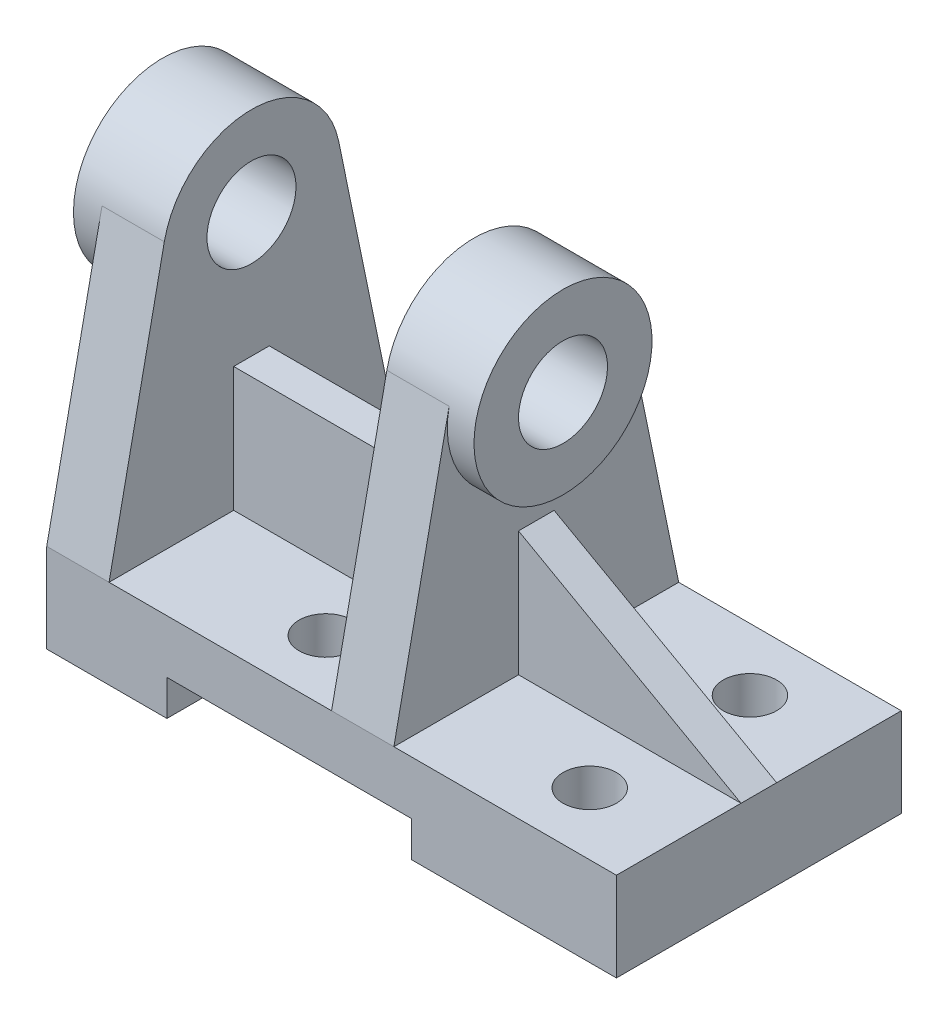
ISO-10303-21;
HEADER;
FILE_DESCRIPTION(('STEP AP214'),'2;1');
FILE_NAME('part.step','',(''),(''),'','','');
FILE_SCHEMA(('AUTOMOTIVE_DESIGN { 1 0 10303 214 1 1 1 1 }'));
ENDSEC;
DATA;
#1=APPLICATION_CONTEXT('core data for automotive mechanical design processes');
#2=APPLICATION_PROTOCOL_DEFINITION('international standard','automotive_design',2000,#1);
#3=PRODUCT_CONTEXT('',#1,'mechanical');
#4=PRODUCT('Part','Part','',(#3));
#5=PRODUCT_RELATED_PRODUCT_CATEGORY('part','',(#4));
#6=PRODUCT_DEFINITION_FORMATION('','',#4);
#7=PRODUCT_DEFINITION_CONTEXT('part definition',#1,'design');
#8=PRODUCT_DEFINITION('design','',#6,#7);
#9=PRODUCT_DEFINITION_SHAPE('','',#8);
#10=(LENGTH_UNIT() NAMED_UNIT(*) SI_UNIT(.MILLI.,.METRE.));
#11=(NAMED_UNIT(*) PLANE_ANGLE_UNIT() SI_UNIT($,.RADIAN.));
#12=(NAMED_UNIT(*) SI_UNIT($,.STERADIAN.) SOLID_ANGLE_UNIT());
#13=UNCERTAINTY_MEASURE_WITH_UNIT(LENGTH_MEASURE(1.E-05),#10,'distance_accuracy_value','');
#14=(GEOMETRIC_REPRESENTATION_CONTEXT(3) GLOBAL_UNCERTAINTY_ASSIGNED_CONTEXT((#13)) GLOBAL_UNIT_ASSIGNED_CONTEXT((#10,
#11,#12)) REPRESENTATION_CONTEXT('',''));
#15=CARTESIAN_POINT('',(0.,0.,0.));
#16=DIRECTION('',(0.,0.,1.));
#17=DIRECTION('',(1.,0.,0.));
#18=AXIS2_PLACEMENT_3D('',#15,#16,#17);
#19=CARTESIAN_POINT('',(78.,28.,-64.));
#20=DIRECTION('',(0.488603368931843,0.87250601594972,0.));
#21=DIRECTION('',(-0.87250601594972,0.488603368931843,0.));
#22=AXIS2_PLACEMENT_3D('',#19,#20,#21);
#23=PLANE('',#22);
#24=DIRECTION('',(0.87250601594972,-0.488603368931843,0.));
#25=VECTOR('',#24,1.);
#26=CARTESIAN_POINT('',(78.,28.,-36.));
#27=LINE('',#26,#25);
#28=CARTESIAN_POINT('',(78.,28.,-36.));
#29=VERTEX_POINT('',#28);
#30=CARTESIAN_POINT('',(128.,0.,-36.));
#31=VERTEX_POINT('',#30);
#32=EDGE_CURVE('E205',#29,#31,#27,.T.);
#33=ORIENTED_EDGE('',*,*,#32,.F.);
#34=DIRECTION('',(0.,0.,1.));
#35=VECTOR('',#34,1.);
#36=CARTESIAN_POINT('',(78.,28.,-64.));
#37=LINE('',#36,#35);
#38=CARTESIAN_POINT('',(78.,28.,-28.));
#39=VERTEX_POINT('',#38);
#40=EDGE_CURVE('E229',#29,#39,#37,.T.);
#41=ORIENTED_EDGE('',*,*,#40,.T.);
#42=DIRECTION('',(-0.87250601594972,0.488603368931843,0.));
#43=VECTOR('',#42,1.);
#44=CARTESIAN_POINT('',(128.,0.,-28.));
#45=LINE('',#44,#43);
#46=CARTESIAN_POINT('',(128.,0.,-28.));
#47=VERTEX_POINT('',#46);
#48=EDGE_CURVE('E220',#47,#39,#45,.T.);
#49=ORIENTED_EDGE('',*,*,#48,.F.);
#50=DIRECTION('',(0.,0.,1.));
#51=VECTOR('',#50,1.);
#52=CARTESIAN_POINT('',(128.,0.,-64.));
#53=LINE('',#52,#51);
#54=EDGE_CURVE('E59',#31,#47,#53,.T.);
#55=ORIENTED_EDGE('',*,*,#54,.F.);
#56=EDGE_LOOP('',(#33,#41,#49,#55));
#57=FACE_BOUND('',#56,.T.);
#58=ADVANCED_FACE('F41',(#57),#23,.T.);
#59=CARTESIAN_POINT('',(78.,56.,-32.));
#60=DIRECTION('',(1.,0.,0.));
#61=DIRECTION('',(0.,1.,0.));
#62=AXIS2_PLACEMENT_3D('',#59,#60,#61);
#63=PLANE('',#62);
#64=ORIENTED_EDGE('',*,*,#40,.F.);
#65=DIRECTION('',(0.,1.,0.));
#66=VECTOR('',#65,1.);
#67=CARTESIAN_POINT('',(78.,0.,-36.));
#68=LINE('',#67,#66);
#69=CARTESIAN_POINT('',(78.,0.,-36.));
#70=VERTEX_POINT('',#69);
#71=EDGE_CURVE('E208',#70,#29,#68,.T.);
#72=ORIENTED_EDGE('',*,*,#71,.F.);
#73=DIRECTION('',(0.,0.,-1.));
#74=VECTOR('',#73,1.);
#75=CARTESIAN_POINT('',(78.,0.,-36.));
#76=LINE('',#75,#74);
#77=CARTESIAN_POINT('',(78.,0.,-64.));
#78=VERTEX_POINT('',#77);
#79=EDGE_CURVE('E211',#70,#78,#76,.T.);
#80=ORIENTED_EDGE('',*,*,#79,.T.);
#81=DIRECTION('',(0.,0.979292061671471,0.202452606669412));
#82=VECTOR('',#81,1.);
#83=CARTESIAN_POINT('',(78.,0.,-64.));
#84=LINE('',#83,#82);
#85=CARTESIAN_POINT('',(78.,60.0490521333883,-51.5858412334294));
#86=VERTEX_POINT('',#85);
#87=EDGE_CURVE('E246',#78,#86,#84,.T.);
#88=ORIENTED_EDGE('',*,*,#87,.T.);
#89=CARTESIAN_POINT('',(78.,56.,-32.));
#90=DIRECTION('',(1.,0.,0.));
#91=DIRECTION('',(0.,1.,0.));
#92=AXIS2_PLACEMENT_3D('',#89,#90,#91);
#93=CIRCLE('',#92,20.);
#94=CARTESIAN_POINT('',(78.,60.0490521333883,-12.4141587665706));
#95=VERTEX_POINT('',#94);
#96=EDGE_CURVE('E243',#95,#86,#93,.T.);
#97=ORIENTED_EDGE('',*,*,#96,.F.);
#98=DIRECTION('',(0.,-0.979292061671471,0.202452606669412));
#99=VECTOR('',#98,1.);
#100=CARTESIAN_POINT('',(78.,0.,0.));
#101=LINE('',#100,#99);
#102=CARTESIAN_POINT('',(78.,0.,0.));
#103=VERTEX_POINT('',#102);
#104=EDGE_CURVE('E253',#95,#103,#101,.T.);
#105=ORIENTED_EDGE('',*,*,#104,.T.);
#106=DIRECTION('',(0.,0.,1.));
#107=VECTOR('',#106,1.);
#108=CARTESIAN_POINT('',(78.,0.,-28.));
#109=LINE('',#108,#107);
#110=CARTESIAN_POINT('',(78.,0.,-28.));
#111=VERTEX_POINT('',#110);
#112=EDGE_CURVE('E223',#111,#103,#109,.T.);
#113=ORIENTED_EDGE('',*,*,#112,.F.);
#114=DIRECTION('',(0.,-1.,0.));
#115=VECTOR('',#114,1.);
#116=CARTESIAN_POINT('',(78.,28.,-28.));
#117=LINE('',#116,#115);
#118=EDGE_CURVE('E219',#39,#111,#117,.T.);
#119=ORIENTED_EDGE('',*,*,#118,.F.);
#120=EDGE_LOOP('',(#64,#72,#80,#88,#97,#105,#113,#119));
#121=FACE_BOUND('',#120,.T.);
#122=ADVANCED_FACE('F462',(#121),#63,.T.);
#123=CARTESIAN_POINT('',(0.,0.,-64.));
#124=DIRECTION('',(0.,1.,0.));
#125=DIRECTION('',(0.,0.,1.));
#126=AXIS2_PLACEMENT_3D('',#123,#124,#125);
#127=PLANE('',#126);
#128=CARTESIAN_POINT('',(48.7,0.,-14.));
#129=DIRECTION('',(0.,1.,0.));
#130=DIRECTION('',(0.,0.,1.));
#131=AXIS2_PLACEMENT_3D('',#128,#129,#130);
#132=CIRCLE('',#131,6.);
#133=CARTESIAN_POINT('',(48.7,0.,-8.00000000000001));
#134=VERTEX_POINT('',#133);
#135=EDGE_CURVE('E561',#134,#134,#132,.T.);
#136=ORIENTED_EDGE('',*,*,#135,.F.);
#137=EDGE_LOOP('',(#136));
#138=FACE_BOUND('',#137,.T.);
#139=DIRECTION('',(-1.,0.,0.));
#140=VECTOR('',#139,1.);
#141=CARTESIAN_POINT('',(0.,0.,0.));
#142=LINE('',#141,#140);
#143=CARTESIAN_POINT('',(64.,0.,0.));
#144=VERTEX_POINT('',#143);
#145=CARTESIAN_POINT('',(14.,0.,0.));
#146=VERTEX_POINT('',#145);
#147=EDGE_CURVE('E174',#144,#146,#142,.T.);
#148=ORIENTED_EDGE('',*,*,#147,.F.);
#149=DIRECTION('',(0.,0.,-1.));
#150=VECTOR('',#149,1.);
#151=CARTESIAN_POINT('',(64.,0.,0.));
#152=LINE('',#151,#150);
#153=CARTESIAN_POINT('',(64.,0.,-28.));
#154=VERTEX_POINT('',#153);
#155=EDGE_CURVE('E258',#144,#154,#152,.T.);
#156=ORIENTED_EDGE('',*,*,#155,.T.);
#157=DIRECTION('',(1.,0.,0.));
#158=VECTOR('',#157,1.);
#159=CARTESIAN_POINT('',(14.,0.,-28.));
#160=LINE('',#159,#158);
#161=CARTESIAN_POINT('',(14.,0.,-28.));
#162=VERTEX_POINT('',#161);
#163=EDGE_CURVE('E297',#162,#154,#160,.T.);
#164=ORIENTED_EDGE('',*,*,#163,.F.);
#165=DIRECTION('',(0.,0.,1.));
#166=VECTOR('',#165,1.);
#167=CARTESIAN_POINT('',(14.,0.,-28.));
#168=LINE('',#167,#166);
#169=EDGE_CURVE('E302',#162,#146,#168,.T.);
#170=ORIENTED_EDGE('',*,*,#169,.T.);
#171=EDGE_LOOP('',(#148,#156,#164,#170));
#172=FACE_BOUND('',#171,.T.);
#173=ADVANCED_FACE('F467',(#138,#172),#127,.T.);
#174=CARTESIAN_POINT('',(48.7,0.,-50.));
#175=DIRECTION('',(0.,1.,0.));
#176=DIRECTION('',(0.,0.,1.));
#177=AXIS2_PLACEMENT_3D('',#174,#175,#176);
#178=CIRCLE('',#177,5.99999999999999);
#179=CARTESIAN_POINT('',(48.7,0.,-44.));
#180=VERTEX_POINT('',#179);
#181=EDGE_CURVE('E196',#180,#180,#178,.T.);
#182=ORIENTED_EDGE('',*,*,#181,.F.);
#183=EDGE_LOOP('',(#182));
#184=FACE_BOUND('',#183,.T.);
#185=DIRECTION('',(-1.,0.,0.));
#186=VECTOR('',#185,1.);
#187=CARTESIAN_POINT('',(64.,0.,-36.));
#188=LINE('',#187,#186);
#189=CARTESIAN_POINT('',(64.,0.,-36.));
#190=VERTEX_POINT('',#189);
#191=CARTESIAN_POINT('',(14.,0.,-36.));
#192=VERTEX_POINT('',#191);
#193=EDGE_CURVE('E282',#190,#192,#188,.T.);
#194=ORIENTED_EDGE('',*,*,#193,.F.);
#195=CARTESIAN_POINT('',(64.,0.,-64.));
#196=VERTEX_POINT('',#195);
#197=EDGE_CURVE('E244',#190,#196,#152,.T.);
#198=ORIENTED_EDGE('',*,*,#197,.T.);
#199=DIRECTION('',(-1.,0.,0.));
#200=VECTOR('',#199,1.);
#201=CARTESIAN_POINT('',(82.,0.,-64.));
#202=LINE('',#201,#200);
#203=CARTESIAN_POINT('',(14.,0.,-64.));
#204=VERTEX_POINT('',#203);
#205=EDGE_CURVE('E154',#196,#204,#202,.T.);
#206=ORIENTED_EDGE('',*,*,#205,.T.);
#207=DIRECTION('',(0.,0.,-1.));
#208=VECTOR('',#207,1.);
#209=CARTESIAN_POINT('',(14.,0.,-36.));
#210=LINE('',#209,#208);
#211=EDGE_CURVE('E287',#192,#204,#210,.T.);
#212=ORIENTED_EDGE('',*,*,#211,.F.);
#213=EDGE_LOOP('',(#194,#198,#206,#212));
#214=FACE_BOUND('',#213,.T.);
#215=ADVANCED_FACE('F511',(#184,#214),#127,.T.);
#216=CARTESIAN_POINT('',(14.,28.,-64.));
#217=DIRECTION('',(0.,1.,0.));
#218=DIRECTION('',(0.,0.,1.));
#219=AXIS2_PLACEMENT_3D('',#216,#217,#218);
#220=PLANE('',#219);
#221=DIRECTION('',(0.,0.,1.));
#222=VECTOR('',#221,1.);
#223=CARTESIAN_POINT('',(64.,28.,-64.));
#224=LINE('',#223,#222);
#225=CARTESIAN_POINT('',(64.,28.,-36.));
#226=VERTEX_POINT('',#225);
#227=CARTESIAN_POINT('',(64.,28.,-28.));
#228=VERTEX_POINT('',#227);
#229=EDGE_CURVE('E306',#226,#228,#224,.T.);
#230=ORIENTED_EDGE('',*,*,#229,.F.);
#231=DIRECTION('',(1.,0.,0.));
#232=VECTOR('',#231,1.);
#233=CARTESIAN_POINT('',(14.,28.,-36.));
#234=LINE('',#233,#232);
#235=CARTESIAN_POINT('',(14.,28.,-36.));
#236=VERTEX_POINT('',#235);
#237=EDGE_CURVE('E279',#236,#226,#234,.T.);
#238=ORIENTED_EDGE('',*,*,#237,.F.);
#239=DIRECTION('',(0.,0.,-1.));
#240=VECTOR('',#239,1.);
#241=CARTESIAN_POINT('',(14.,28.,0.));
#242=LINE('',#241,#240);
#243=CARTESIAN_POINT('',(14.,28.,-28.));
#244=VERTEX_POINT('',#243);
#245=EDGE_CURVE('E11',#244,#236,#242,.T.);
#246=ORIENTED_EDGE('',*,*,#245,.F.);
#247=DIRECTION('',(-1.,0.,0.));
#248=VECTOR('',#247,1.);
#249=CARTESIAN_POINT('',(64.,28.,-28.));
#250=LINE('',#249,#248);
#251=EDGE_CURVE('E291',#228,#244,#250,.T.);
#252=ORIENTED_EDGE('',*,*,#251,.F.);
#253=EDGE_LOOP('',(#230,#238,#246,#252));
#254=FACE_BOUND('',#253,.T.);
#255=ADVANCED_FACE('F507',(#254),#220,.T.);
#256=CARTESIAN_POINT('',(0.,0.,-64.));
#257=DIRECTION('',(-1.,0.,0.));
#258=DIRECTION('',(0.,0.,1.));
#259=AXIS2_PLACEMENT_3D('',#256,#257,#258);
#260=PLANE('',#259);
#261=CARTESIAN_POINT('',(0.,56.,-32.));
#262=DIRECTION('',(-1.,0.,0.));
#263=DIRECTION('',(0.,0.,1.));
#264=AXIS2_PLACEMENT_3D('',#261,#262,#263);
#265=CIRCLE('',#264,20.);
#266=CARTESIAN_POINT('',(0.,60.0490521333882,-51.5858412334294));
#267=VERTEX_POINT('',#266);
#268=CARTESIAN_POINT('',(0.,60.0490521333882,-12.4141587665706));
#269=VERTEX_POINT('',#268);
#270=EDGE_CURVE('E49',#267,#269,#265,.T.);
#271=ORIENTED_EDGE('',*,*,#270,.F.);
#272=DIRECTION('',(0.,0.979292061671471,0.202452606669412));
#273=VECTOR('',#272,1.);
#274=CARTESIAN_POINT('',(0.,12.6886547568673,-61.3768282913767));
#275=LINE('',#274,#273);
#276=CARTESIAN_POINT('',(0.,0.,-64.));
#277=VERTEX_POINT('',#276);
#278=EDGE_CURVE('E330',#277,#267,#275,.T.);
#279=ORIENTED_EDGE('',*,*,#278,.F.);
#280=DIRECTION('',(0.,-1.,0.));
#281=VECTOR('',#280,1.);
#282=CARTESIAN_POINT('',(0.,0.,-64.));
#283=LINE('',#282,#281);
#284=CARTESIAN_POINT('',(0.,-20.,-64.));
#285=VERTEX_POINT('',#284);
#286=EDGE_CURVE('E70',#277,#285,#283,.T.);
#287=ORIENTED_EDGE('',*,*,#286,.T.);
#288=DIRECTION('',(0.,0.,1.));
#289=VECTOR('',#288,1.);
#290=CARTESIAN_POINT('',(0.,-20.,-64.));
#291=LINE('',#290,#289);
#292=CARTESIAN_POINT('',(0.,-20.,0.));
#293=VERTEX_POINT('',#292);
#294=EDGE_CURVE('E110',#285,#293,#291,.T.);
#295=ORIENTED_EDGE('',*,*,#294,.T.);
#296=DIRECTION('',(0.,-1.,0.));
#297=VECTOR('',#296,1.);
#298=CARTESIAN_POINT('',(0.,0.,0.));
#299=LINE('',#298,#297);
#300=CARTESIAN_POINT('',(0.,0.,0.));
#301=VERTEX_POINT('',#300);
#302=EDGE_CURVE('E158',#301,#293,#299,.T.);
#303=ORIENTED_EDGE('',*,*,#302,.F.);
#304=DIRECTION('',(0.,0.979292061671471,-0.202452606669412));
#305=VECTOR('',#304,1.);
#306=CARTESIAN_POINT('',(0.,0.,0.));
#307=LINE('',#306,#305);
#308=EDGE_CURVE('E319',#301,#269,#307,.T.);
#309=ORIENTED_EDGE('',*,*,#308,.T.);
#310=EDGE_LOOP('',(#271,#279,#287,#295,#303,#309));
#311=FACE_BOUND('',#310,.T.);
#312=ADVANCED_FACE('F43',(#311),#260,.T.);
#313=CARTESIAN_POINT('',(128.,0.,-64.));
#314=DIRECTION('',(1.,0.,0.));
#315=DIRECTION('',(0.,0.,-1.));
#316=AXIS2_PLACEMENT_3D('',#313,#314,#315);
#317=PLANE('',#316);
#318=DIRECTION('',(0.,1.,0.));
#319=VECTOR('',#318,1.);
#320=CARTESIAN_POINT('',(128.,0.,0.));
#321=LINE('',#320,#319);
#322=CARTESIAN_POINT('',(128.,-20.,0.));
#323=VERTEX_POINT('',#322);
#324=CARTESIAN_POINT('',(128.,0.,0.));
#325=VERTEX_POINT('',#324);
#326=EDGE_CURVE('E175',#323,#325,#321,.T.);
#327=ORIENTED_EDGE('',*,*,#326,.F.);
#328=DIRECTION('',(0.,0.,1.));
#329=VECTOR('',#328,1.);
#330=CARTESIAN_POINT('',(128.,-20.,-64.));
#331=LINE('',#330,#329);
#332=CARTESIAN_POINT('',(128.,-20.,-64.));
#333=VERTEX_POINT('',#332);
#334=EDGE_CURVE('E131',#333,#323,#331,.T.);
#335=ORIENTED_EDGE('',*,*,#334,.F.);
#336=DIRECTION('',(0.,1.,0.));
#337=VECTOR('',#336,1.);
#338=CARTESIAN_POINT('',(128.,0.,-64.));
#339=LINE('',#338,#337);
#340=CARTESIAN_POINT('',(128.,0.,-64.));
#341=VERTEX_POINT('',#340);
#342=EDGE_CURVE('E144',#333,#341,#339,.T.);
#343=ORIENTED_EDGE('',*,*,#342,.T.);
#344=EDGE_CURVE('E180',#341,#31,#53,.T.);
#345=ORIENTED_EDGE('',*,*,#344,.T.);
#346=ORIENTED_EDGE('',*,*,#54,.T.);
#347=DIRECTION('',(0.,0.,1.));
#348=VECTOR('',#347,1.);
#349=CARTESIAN_POINT('',(128.,0.,-28.));
#350=LINE('',#349,#348);
#351=EDGE_CURVE('E226',#47,#325,#350,.T.);
#352=ORIENTED_EDGE('',*,*,#351,.T.);
#353=EDGE_LOOP('',(#327,#335,#343,#345,#346,#352));
#354=FACE_BOUND('',#353,.T.);
#355=ADVANCED_FACE('F448',(#354),#317,.T.);
#356=CARTESIAN_POINT('',(128.,-20.,-64.));
#357=DIRECTION('',(0.,-1.,0.));
#358=DIRECTION('',(0.,0.,-1.));
#359=AXIS2_PLACEMENT_3D('',#356,#357,#358);
#360=PLANE('',#359);
#361=CARTESIAN_POINT('',(108.,-20.,-14.));
#362=DIRECTION('',(0.,-1.,0.));
#363=DIRECTION('',(0.,0.,-1.));
#364=AXIS2_PLACEMENT_3D('',#361,#362,#363);
#365=CIRCLE('',#364,6.);
#366=CARTESIAN_POINT('',(108.,-20.,-20.));
#367=VERTEX_POINT('',#366);
#368=EDGE_CURVE('E190',#367,#367,#365,.T.);
#369=ORIENTED_EDGE('',*,*,#368,.F.);
#370=EDGE_LOOP('',(#369));
#371=FACE_BOUND('',#370,.T.);
#372=CARTESIAN_POINT('',(108.,-20.,-50.));
#373=DIRECTION('',(0.,-1.,0.));
#374=DIRECTION('',(0.,0.,-1.));
#375=AXIS2_PLACEMENT_3D('',#372,#373,#374);
#376=CIRCLE('',#375,6.);
#377=CARTESIAN_POINT('',(108.,-20.,-56.));
#378=VERTEX_POINT('',#377);
#379=EDGE_CURVE('E191',#378,#378,#376,.T.);
#380=ORIENTED_EDGE('',*,*,#379,.F.);
#381=EDGE_LOOP('',(#380));
#382=FACE_BOUND('',#381,.T.);
#383=DIRECTION('',(1.,0.,0.));
#384=VECTOR('',#383,1.);
#385=CARTESIAN_POINT('',(128.,-20.,0.));
#386=LINE('',#385,#384);
#387=CARTESIAN_POINT('',(82.,-20.,0.));
#388=VERTEX_POINT('',#387);
#389=EDGE_CURVE('E126',#388,#323,#386,.T.);
#390=ORIENTED_EDGE('',*,*,#389,.F.);
#391=DIRECTION('',(0.,0.,1.));
#392=VECTOR('',#391,1.);
#393=CARTESIAN_POINT('',(82.,-20.,-64.));
#394=LINE('',#393,#392);
#395=CARTESIAN_POINT('',(82.,-20.,-64.));
#396=VERTEX_POINT('',#395);
#397=EDGE_CURVE('E121',#396,#388,#394,.T.);
#398=ORIENTED_EDGE('',*,*,#397,.F.);
#399=DIRECTION('',(1.,0.,0.));
#400=VECTOR('',#399,1.);
#401=CARTESIAN_POINT('',(128.,-20.,-64.));
#402=LINE('',#401,#400);
#403=EDGE_CURVE('E127',#396,#333,#402,.T.);
#404=ORIENTED_EDGE('',*,*,#403,.T.);
#405=ORIENTED_EDGE('',*,*,#334,.T.);
#406=EDGE_LOOP('',(#390,#398,#404,#405));
#407=FACE_BOUND('',#406,.T.);
#408=ADVANCED_FACE('F122',(#371,#382,#407),#360,.T.);
#409=CARTESIAN_POINT('',(82.,-12.,-64.));
#410=DIRECTION('',(-1.,0.,0.));
#411=DIRECTION('',(0.,0.,1.));
#412=AXIS2_PLACEMENT_3D('',#409,#410,#411);
#413=PLANE('',#412);
#414=DIRECTION('',(0.,-1.,0.));
#415=VECTOR('',#414,1.);
#416=CARTESIAN_POINT('',(82.,-12.,0.));
#417=LINE('',#416,#415);
#418=CARTESIAN_POINT('',(82.,-12.,0.));
#419=VERTEX_POINT('',#418);
#420=EDGE_CURVE('E166',#419,#388,#417,.T.);
#421=ORIENTED_EDGE('',*,*,#420,.F.);
#422=DIRECTION('',(0.,0.,1.));
#423=VECTOR('',#422,1.);
#424=CARTESIAN_POINT('',(82.,-12.,-64.));
#425=LINE('',#424,#423);
#426=CARTESIAN_POINT('',(82.,-12.,-64.));
#427=VERTEX_POINT('',#426);
#428=EDGE_CURVE('E132',#427,#419,#425,.T.);
#429=ORIENTED_EDGE('',*,*,#428,.F.);
#430=DIRECTION('',(0.,-1.,0.));
#431=VECTOR('',#430,1.);
#432=CARTESIAN_POINT('',(82.,-12.,-64.));
#433=LINE('',#432,#431);
#434=EDGE_CURVE('E143',#427,#396,#433,.T.);
#435=ORIENTED_EDGE('',*,*,#434,.T.);
#436=ORIENTED_EDGE('',*,*,#397,.T.);
#437=EDGE_LOOP('',(#421,#429,#435,#436));
#438=FACE_BOUND('',#437,.T.);
#439=ADVANCED_FACE('F150',(#438),#413,.T.);
#440=CARTESIAN_POINT('',(27.,-12.,-64.));
#441=DIRECTION('',(0.,-1.,0.));
#442=DIRECTION('',(0.,0.,-1.));
#443=AXIS2_PLACEMENT_3D('',#440,#441,#442);
#444=PLANE('',#443);
#445=CARTESIAN_POINT('',(48.7,-12.,-14.));
#446=DIRECTION('',(0.,-1.,0.));
#447=DIRECTION('',(0.,0.,-1.));
#448=AXIS2_PLACEMENT_3D('',#445,#446,#447);
#449=CIRCLE('',#448,6.);
#450=CARTESIAN_POINT('',(48.7,-12.,-20.));
#451=VERTEX_POINT('',#450);
#452=EDGE_CURVE('E44',#451,#451,#449,.T.);
#453=ORIENTED_EDGE('',*,*,#452,.F.);
#454=EDGE_LOOP('',(#453));
#455=FACE_BOUND('',#454,.T.);
#456=CARTESIAN_POINT('',(48.7,-12.,-50.));
#457=DIRECTION('',(0.,-1.,0.));
#458=DIRECTION('',(0.,0.,-1.));
#459=AXIS2_PLACEMENT_3D('',#456,#457,#458);
#460=CIRCLE('',#459,5.99999999999999);
#461=CARTESIAN_POINT('',(48.7,-12.,-56.));
#462=VERTEX_POINT('',#461);
#463=EDGE_CURVE('E183',#462,#462,#460,.T.);
#464=ORIENTED_EDGE('',*,*,#463,.F.);
#465=EDGE_LOOP('',(#464));
#466=FACE_BOUND('',#465,.T.);
#467=DIRECTION('',(1.,0.,0.));
#468=VECTOR('',#467,1.);
#469=CARTESIAN_POINT('',(27.,-12.,0.));
#470=LINE('',#469,#468);
#471=CARTESIAN_POINT('',(27.,-12.,0.));
#472=VERTEX_POINT('',#471);
#473=EDGE_CURVE('E167',#472,#419,#470,.T.);
#474=ORIENTED_EDGE('',*,*,#473,.F.);
#475=DIRECTION('',(0.,0.,1.));
#476=VECTOR('',#475,1.);
#477=CARTESIAN_POINT('',(27.,-12.,-64.));
#478=LINE('',#477,#476);
#479=CARTESIAN_POINT('',(27.,-12.,-64.));
#480=VERTEX_POINT('',#479);
#481=EDGE_CURVE('E182',#480,#472,#478,.T.);
#482=ORIENTED_EDGE('',*,*,#481,.F.);
#483=DIRECTION('',(1.,0.,0.));
#484=VECTOR('',#483,1.);
#485=CARTESIAN_POINT('',(27.,-12.,-64.));
#486=LINE('',#485,#484);
#487=EDGE_CURVE('E146',#480,#427,#486,.T.);
#488=ORIENTED_EDGE('',*,*,#487,.T.);
#489=ORIENTED_EDGE('',*,*,#428,.T.);
#490=EDGE_LOOP('',(#474,#482,#488,#489));
#491=FACE_BOUND('',#490,.T.);
#492=ADVANCED_FACE('F447',(#455,#466,#491),#444,.T.);
#493=CARTESIAN_POINT('',(27.,-20.,-64.));
#494=DIRECTION('',(1.,0.,0.));
#495=DIRECTION('',(0.,0.,-1.));
#496=AXIS2_PLACEMENT_3D('',#493,#494,#495);
#497=PLANE('',#496);
#498=DIRECTION('',(0.,1.,0.));
#499=VECTOR('',#498,1.);
#500=CARTESIAN_POINT('',(27.,-20.,0.));
#501=LINE('',#500,#499);
#502=CARTESIAN_POINT('',(27.,-20.,0.));
#503=VERTEX_POINT('',#502);
#504=EDGE_CURVE('E162',#503,#472,#501,.T.);
#505=ORIENTED_EDGE('',*,*,#504,.F.);
#506=DIRECTION('',(0.,0.,1.));
#507=VECTOR('',#506,1.);
#508=CARTESIAN_POINT('',(27.,-20.,-64.));
#509=LINE('',#508,#507);
#510=CARTESIAN_POINT('',(27.,-20.,-64.));
#511=VERTEX_POINT('',#510);
#512=EDGE_CURVE('E181',#511,#503,#509,.T.);
#513=ORIENTED_EDGE('',*,*,#512,.F.);
#514=DIRECTION('',(0.,1.,0.));
#515=VECTOR('',#514,1.);
#516=CARTESIAN_POINT('',(27.,-20.,-64.));
#517=LINE('',#516,#515);
#518=EDGE_CURVE('E147',#511,#480,#517,.T.);
#519=ORIENTED_EDGE('',*,*,#518,.T.);
#520=ORIENTED_EDGE('',*,*,#481,.T.);
#521=EDGE_LOOP('',(#505,#513,#519,#520));
#522=FACE_BOUND('',#521,.T.);
#523=ADVANCED_FACE('F355',(#522),#497,.T.);
#524=CARTESIAN_POINT('',(0.,-20.,-64.));
#525=DIRECTION('',(0.,-1.,0.));
#526=DIRECTION('',(0.,0.,-1.));
#527=AXIS2_PLACEMENT_3D('',#524,#525,#526);
#528=PLANE('',#527);
#529=DIRECTION('',(1.,0.,0.));
#530=VECTOR('',#529,1.);
#531=CARTESIAN_POINT('',(0.,-20.,0.));
#532=LINE('',#531,#530);
#533=EDGE_CURVE('E159',#293,#503,#532,.T.);
#534=ORIENTED_EDGE('',*,*,#533,.F.);
#535=ORIENTED_EDGE('',*,*,#294,.F.);
#536=DIRECTION('',(1.,0.,0.));
#537=VECTOR('',#536,1.);
#538=CARTESIAN_POINT('',(0.,-20.,-64.));
#539=LINE('',#538,#537);
#540=EDGE_CURVE('E350',#285,#511,#539,.T.);
#541=ORIENTED_EDGE('',*,*,#540,.T.);
#542=ORIENTED_EDGE('',*,*,#512,.T.);
#543=EDGE_LOOP('',(#534,#535,#541,#542));
#544=FACE_BOUND('',#543,.T.);
#545=ADVANCED_FACE('F352',(#544),#528,.T.);
#546=CARTESIAN_POINT('',(0.,0.,-64.));
#547=DIRECTION('',(0.,0.,1.));
#548=DIRECTION('',(1.,0.,0.));
#549=AXIS2_PLACEMENT_3D('',#546,#547,#548);
#550=PLANE('',#549);
#551=DIRECTION('',(-1.,0.,0.));
#552=VECTOR('',#551,1.);
#553=CARTESIAN_POINT('',(78.,0.,-64.));
#554=LINE('',#553,#552);
#555=EDGE_CURVE('E274',#78,#196,#554,.T.);
#556=ORIENTED_EDGE('',*,*,#555,.F.);
#557=DIRECTION('',(-1.,0.,0.));
#558=VECTOR('',#557,1.);
#559=CARTESIAN_POINT('',(128.,0.,-64.));
#560=LINE('',#559,#558);
#561=EDGE_CURVE('E193',#341,#78,#560,.T.);
#562=ORIENTED_EDGE('',*,*,#561,.F.);
#563=ORIENTED_EDGE('',*,*,#342,.F.);
#564=ORIENTED_EDGE('',*,*,#403,.F.);
#565=ORIENTED_EDGE('',*,*,#434,.F.);
#566=ORIENTED_EDGE('',*,*,#487,.F.);
#567=ORIENTED_EDGE('',*,*,#518,.F.);
#568=ORIENTED_EDGE('',*,*,#540,.F.);
#569=ORIENTED_EDGE('',*,*,#286,.F.);
#570=DIRECTION('',(-1.,0.,0.));
#571=VECTOR('',#570,1.);
#572=CARTESIAN_POINT('',(14.,0.,-64.));
#573=LINE('',#572,#571);
#574=EDGE_CURVE('E337',#204,#277,#573,.T.);
#575=ORIENTED_EDGE('',*,*,#574,.F.);
#576=ORIENTED_EDGE('',*,*,#205,.F.);
#577=EDGE_LOOP('',(#556,#562,#563,#564,#565,#566,#567,#568,#569,#575,#576));
#578=FACE_BOUND('',#577,.T.);
#579=ADVANCED_FACE('F139',(#578),#550,.F.);
#580=CARTESIAN_POINT('',(0.,0.,0.));
#581=DIRECTION('',(0.,0.,1.));
#582=DIRECTION('',(1.,0.,0.));
#583=AXIS2_PLACEMENT_3D('',#580,#581,#582);
#584=PLANE('',#583);
#585=DIRECTION('',(1.,0.,0.));
#586=VECTOR('',#585,1.);
#587=CARTESIAN_POINT('',(78.,0.,0.));
#588=LINE('',#587,#586);
#589=EDGE_CURVE('E216',#103,#325,#588,.T.);
#590=ORIENTED_EDGE('',*,*,#589,.F.);
#591=DIRECTION('',(-1.,0.,0.));
#592=VECTOR('',#591,1.);
#593=CARTESIAN_POINT('',(78.,0.,0.));
#594=LINE('',#593,#592);
#595=EDGE_CURVE('E254',#103,#144,#594,.T.);
#596=ORIENTED_EDGE('',*,*,#595,.T.);
#597=ORIENTED_EDGE('',*,*,#147,.T.);
#598=DIRECTION('',(-1.,0.,0.));
#599=VECTOR('',#598,1.);
#600=CARTESIAN_POINT('',(14.,0.,0.));
#601=LINE('',#600,#599);
#602=EDGE_CURVE('E97',#146,#301,#601,.T.);
#603=ORIENTED_EDGE('',*,*,#602,.T.);
#604=ORIENTED_EDGE('',*,*,#302,.T.);
#605=ORIENTED_EDGE('',*,*,#533,.T.);
#606=ORIENTED_EDGE('',*,*,#504,.T.);
#607=ORIENTED_EDGE('',*,*,#473,.T.);
#608=ORIENTED_EDGE('',*,*,#420,.T.);
#609=ORIENTED_EDGE('',*,*,#389,.T.);
#610=ORIENTED_EDGE('',*,*,#326,.T.);
#611=EDGE_LOOP('',(#590,#596,#597,#603,#604,#605,#606,#607,#608,#609,#610));
#612=FACE_BOUND('',#611,.T.);
#613=ADVANCED_FACE('F358',(#612),#584,.T.);
#614=CARTESIAN_POINT('',(14.,0.,0.));
#615=DIRECTION('',(0.,0.202452606669412,0.979292061671471));
#616=DIRECTION('',(0.,-0.979292061671471,0.202452606669412));
#617=AXIS2_PLACEMENT_3D('',#614,#615,#616);
#618=PLANE('',#617);
#619=ORIENTED_EDGE('',*,*,#308,.F.);
#620=ORIENTED_EDGE('',*,*,#602,.F.);
#621=DIRECTION('',(0.,0.979292061671471,-0.202452606669412));
#622=VECTOR('',#621,1.);
#623=CARTESIAN_POINT('',(14.,0.,0.));
#624=LINE('',#623,#622);
#625=CARTESIAN_POINT('',(14.,60.0490521333882,-12.4141587665706));
#626=VERTEX_POINT('',#625);
#627=EDGE_CURVE('E323',#146,#626,#624,.T.);
#628=ORIENTED_EDGE('',*,*,#627,.T.);
#629=DIRECTION('',(-1.,0.,0.));
#630=VECTOR('',#629,1.);
#631=CARTESIAN_POINT('',(14.,60.0490521333882,-12.4141587665706));
#632=LINE('',#631,#630);
#633=EDGE_CURVE('E334',#626,#269,#632,.T.);
#634=ORIENTED_EDGE('',*,*,#633,.T.);
#635=EDGE_LOOP('',(#619,#620,#628,#634));
#636=FACE_BOUND('',#635,.T.);
#637=ADVANCED_FACE('F362',(#636),#618,.T.);
#638=CARTESIAN_POINT('',(14.,12.6886547568673,-61.3768282913767));
#639=DIRECTION('',(0.,-0.202452606669412,0.979292061671471));
#640=DIRECTION('',(0.,-0.979292061671471,-0.202452606669412));
#641=AXIS2_PLACEMENT_3D('',#638,#639,#640);
#642=PLANE('',#641);
#643=ORIENTED_EDGE('',*,*,#278,.T.);
#644=DIRECTION('',(-1.,0.,0.));
#645=VECTOR('',#644,1.);
#646=CARTESIAN_POINT('',(14.,60.0490521333882,-51.5858412334294));
#647=LINE('',#646,#645);
#648=CARTESIAN_POINT('',(14.,60.0490521333882,-51.5858412334294));
#649=VERTEX_POINT('',#648);
#650=EDGE_CURVE('E343',#649,#267,#647,.T.);
#651=ORIENTED_EDGE('',*,*,#650,.F.);
#652=DIRECTION('',(0.,0.979292061671471,0.202452606669412));
#653=VECTOR('',#652,1.);
#654=CARTESIAN_POINT('',(14.,12.6886547568673,-61.3768282913767));
#655=LINE('',#654,#653);
#656=EDGE_CURVE('E329',#204,#649,#655,.T.);
#657=ORIENTED_EDGE('',*,*,#656,.F.);
#658=ORIENTED_EDGE('',*,*,#574,.T.);
#659=EDGE_LOOP('',(#643,#651,#657,#658));
#660=FACE_BOUND('',#659,.T.);
#661=ADVANCED_FACE('F528',(#660),#642,.F.);
#662=CARTESIAN_POINT('',(14.,56.,-32.));
#663=DIRECTION('',(-1.,0.,0.));
#664=DIRECTION('',(0.,0.,1.));
#665=AXIS2_PLACEMENT_3D('',#662,#663,#664);
#666=CYLINDRICAL_SURFACE('',#665,20.);
#667=ORIENTED_EDGE('',*,*,#650,.T.);
#668=ORIENTED_EDGE('',*,*,#270,.T.);
#669=ORIENTED_EDGE('',*,*,#633,.F.);
#670=CARTESIAN_POINT('',(14.,56.,-32.));
#671=DIRECTION('',(-1.,0.,0.));
#672=DIRECTION('',(0.,0.,1.));
#673=AXIS2_PLACEMENT_3D('',#670,#671,#672);
#674=CIRCLE('',#673,20.);
#675=EDGE_CURVE('E326',#626,#649,#674,.T.);
#676=ORIENTED_EDGE('',*,*,#675,.T.);
#677=EDGE_LOOP('',(#667,#668,#669,#676));
#678=FACE_BOUND('',#677,.T.);
#679=CARTESIAN_POINT('',(-6.,56.,-32.));
#680=DIRECTION('',(-1.,0.,0.));
#681=DIRECTION('',(0.,0.,1.));
#682=AXIS2_PLACEMENT_3D('',#679,#680,#681);
#683=CIRCLE('',#682,20.);
#684=CARTESIAN_POINT('',(-6.,56.,-12.));
#685=VERTEX_POINT('',#684);
#686=EDGE_CURVE('E320',#685,#685,#683,.T.);
#687=ORIENTED_EDGE('',*,*,#686,.F.);
#688=EDGE_LOOP('',(#687));
#689=FACE_BOUND('',#688,.T.);
#690=ADVANCED_FACE('F371',(#678,#689),#666,.T.);
#691=CARTESIAN_POINT('',(14.,0.,0.));
#692=DIRECTION('',(-1.,0.,0.));
#693=DIRECTION('',(0.,0.,1.));
#694=AXIS2_PLACEMENT_3D('',#691,#692,#693);
#695=PLANE('',#694);
#696=CARTESIAN_POINT('',(14.,56.,-32.));
#697=DIRECTION('',(-1.,0.,0.));
#698=DIRECTION('',(0.,0.,1.));
#699=AXIS2_PLACEMENT_3D('',#696,#697,#698);
#700=CIRCLE('',#699,10.);
#701=CARTESIAN_POINT('',(14.,56.,-22.));
#702=VERTEX_POINT('',#701);
#703=EDGE_CURVE('E314',#702,#702,#700,.T.);
#704=ORIENTED_EDGE('',*,*,#703,.T.);
#705=EDGE_LOOP('',(#704));
#706=FACE_BOUND('',#705,.T.);
#707=ORIENTED_EDGE('',*,*,#675,.F.);
#708=ORIENTED_EDGE('',*,*,#627,.F.);
#709=ORIENTED_EDGE('',*,*,#169,.F.);
#710=DIRECTION('',(0.,-1.,0.));
#711=VECTOR('',#710,1.);
#712=CARTESIAN_POINT('',(14.,28.,-28.));
#713=LINE('',#712,#711);
#714=EDGE_CURVE('E298',#244,#162,#713,.T.);
#715=ORIENTED_EDGE('',*,*,#714,.F.);
#716=ORIENTED_EDGE('',*,*,#245,.T.);
#717=DIRECTION('',(0.,1.,0.));
#718=VECTOR('',#717,1.);
#719=CARTESIAN_POINT('',(14.,0.,-36.));
#720=LINE('',#719,#718);
#721=EDGE_CURVE('E290',#192,#236,#720,.T.);
#722=ORIENTED_EDGE('',*,*,#721,.F.);
#723=ORIENTED_EDGE('',*,*,#211,.T.);
#724=ORIENTED_EDGE('',*,*,#656,.T.);
#725=EDGE_LOOP('',(#707,#708,#709,#715,#716,#722,#723,#724));
#726=FACE_BOUND('',#725,.T.);
#727=ADVANCED_FACE('F523',(#706,#726),#695,.F.);
#728=CARTESIAN_POINT('',(-6.,56.,-32.));
#729=DIRECTION('',(-1.,0.,0.));
#730=DIRECTION('',(0.,0.,1.));
#731=AXIS2_PLACEMENT_3D('',#728,#729,#730);
#732=PLANE('',#731);
#733=CARTESIAN_POINT('',(-6.,56.,-32.));
#734=DIRECTION('',(-1.,0.,0.));
#735=DIRECTION('',(0.,0.,1.));
#736=AXIS2_PLACEMENT_3D('',#733,#734,#735);
#737=CIRCLE('',#736,10.);
#738=CARTESIAN_POINT('',(-6.,56.,-22.));
#739=VERTEX_POINT('',#738);
#740=EDGE_CURVE('E313',#739,#739,#737,.T.);
#741=ORIENTED_EDGE('',*,*,#740,.F.);
#742=EDGE_LOOP('',(#741));
#743=FACE_BOUND('',#742,.T.);
#744=ORIENTED_EDGE('',*,*,#686,.T.);
#745=EDGE_LOOP('',(#744));
#746=FACE_BOUND('',#745,.T.);
#747=ADVANCED_FACE('F520',(#743,#746),#732,.T.);
#748=CARTESIAN_POINT('',(24.,56.,-32.));
#749=DIRECTION('',(-1.,0.,0.));
#750=DIRECTION('',(0.,0.,1.));
#751=AXIS2_PLACEMENT_3D('',#748,#749,#750);
#752=CYLINDRICAL_SURFACE('',#751,10.);
#753=ORIENTED_EDGE('',*,*,#740,.T.);
#754=EDGE_LOOP('',(#753));
#755=FACE_BOUND('',#754,.T.);
#756=ORIENTED_EDGE('',*,*,#703,.F.);
#757=EDGE_LOOP('',(#756));
#758=FACE_BOUND('',#757,.T.);
#759=ADVANCED_FACE('F506',(#755,#758),#752,.F.);
#760=CARTESIAN_POINT('',(0.,0.,-28.));
#761=DIRECTION('',(0.,0.,1.));
#762=DIRECTION('',(1.,0.,0.));
#763=AXIS2_PLACEMENT_3D('',#760,#761,#762);
#764=PLANE('',#763);
#765=ORIENTED_EDGE('',*,*,#251,.T.);
#766=ORIENTED_EDGE('',*,*,#714,.T.);
#767=ORIENTED_EDGE('',*,*,#163,.T.);
#768=DIRECTION('',(0.,1.,0.));
#769=VECTOR('',#768,1.);
#770=CARTESIAN_POINT('',(64.,0.,-28.));
#771=LINE('',#770,#769);
#772=EDGE_CURVE('E305',#154,#228,#771,.T.);
#773=ORIENTED_EDGE('',*,*,#772,.T.);
#774=EDGE_LOOP('',(#765,#766,#767,#773));
#775=FACE_BOUND('',#774,.T.);
#776=ADVANCED_FACE('F502',(#775),#764,.T.);
#777=CARTESIAN_POINT('',(0.,0.,-36.));
#778=DIRECTION('',(0.,0.,-1.));
#779=DIRECTION('',(-1.,0.,0.));
#780=AXIS2_PLACEMENT_3D('',#777,#778,#779);
#781=PLANE('',#780);
#782=ORIENTED_EDGE('',*,*,#237,.T.);
#783=DIRECTION('',(0.,-1.,0.));
#784=VECTOR('',#783,1.);
#785=CARTESIAN_POINT('',(64.,28.,-36.));
#786=LINE('',#785,#784);
#787=EDGE_CURVE('E283',#226,#190,#786,.T.);
#788=ORIENTED_EDGE('',*,*,#787,.T.);
#789=ORIENTED_EDGE('',*,*,#193,.T.);
#790=ORIENTED_EDGE('',*,*,#721,.T.);
#791=EDGE_LOOP('',(#782,#788,#789,#790));
#792=FACE_BOUND('',#791,.T.);
#793=ADVANCED_FACE('F498',(#792),#781,.T.);
#794=CARTESIAN_POINT('',(78.,0.,-64.));
#795=DIRECTION('',(0.,-0.202452606669412,0.979292061671471));
#796=DIRECTION('',(0.,-0.979292061671471,-0.202452606669412));
#797=AXIS2_PLACEMENT_3D('',#794,#795,#796);
#798=PLANE('',#797);
#799=DIRECTION('',(0.,0.979292061671471,0.202452606669412));
#800=VECTOR('',#799,1.);
#801=CARTESIAN_POINT('',(64.,0.,-64.));
#802=LINE('',#801,#800);
#803=CARTESIAN_POINT('',(64.,60.0490521333883,-51.5858412334294));
#804=VERTEX_POINT('',#803);
#805=EDGE_CURVE('E259',#196,#804,#802,.T.);
#806=ORIENTED_EDGE('',*,*,#805,.T.);
#807=DIRECTION('',(-1.,0.,0.));
#808=VECTOR('',#807,1.);
#809=CARTESIAN_POINT('',(78.,60.0490521333883,-51.5858412334294));
#810=LINE('',#809,#808);
#811=EDGE_CURVE('E275',#86,#804,#810,.T.);
#812=ORIENTED_EDGE('',*,*,#811,.F.);
#813=ORIENTED_EDGE('',*,*,#87,.F.);
#814=ORIENTED_EDGE('',*,*,#555,.T.);
#815=EDGE_LOOP('',(#806,#812,#813,#814));
#816=FACE_BOUND('',#815,.T.);
#817=ADVANCED_FACE('F497',(#816),#798,.F.);
#818=CARTESIAN_POINT('',(78.,56.,-32.));
#819=DIRECTION('',(-1.,0.,0.));
#820=DIRECTION('',(0.,-1.,0.));
#821=AXIS2_PLACEMENT_3D('',#818,#819,#820);
#822=CYLINDRICAL_SURFACE('',#821,20.);
#823=CARTESIAN_POINT('',(64.,56.,-32.));
#824=DIRECTION('',(1.,0.,0.));
#825=DIRECTION('',(0.,1.,0.));
#826=AXIS2_PLACEMENT_3D('',#823,#824,#825);
#827=CIRCLE('',#826,20.);
#828=CARTESIAN_POINT('',(64.,60.0490521333883,-12.4141587665706));
#829=VERTEX_POINT('',#828);
#830=EDGE_CURVE('E265',#804,#829,#827,.T.);
#831=ORIENTED_EDGE('',*,*,#830,.T.);
#832=DIRECTION('',(-1.,0.,0.));
#833=VECTOR('',#832,1.);
#834=CARTESIAN_POINT('',(78.,60.0490521333883,-12.4141587665706));
#835=LINE('',#834,#833);
#836=EDGE_CURVE('E267',#95,#829,#835,.T.);
#837=ORIENTED_EDGE('',*,*,#836,.F.);
#838=ORIENTED_EDGE('',*,*,#96,.T.);
#839=ORIENTED_EDGE('',*,*,#811,.T.);
#840=EDGE_LOOP('',(#831,#837,#838,#839));
#841=FACE_BOUND('',#840,.T.);
#842=CARTESIAN_POINT('',(84.,56.,-32.));
#843=DIRECTION('',(1.,0.,0.));
#844=DIRECTION('',(0.,1.,0.));
#845=AXIS2_PLACEMENT_3D('',#842,#843,#844);
#846=CIRCLE('',#845,20.);
#847=CARTESIAN_POINT('',(84.,76.,-32.));
#848=VERTEX_POINT('',#847);
#849=EDGE_CURVE('E245',#848,#848,#846,.T.);
#850=ORIENTED_EDGE('',*,*,#849,.F.);
#851=EDGE_LOOP('',(#850));
#852=FACE_BOUND('',#851,.T.);
#853=ADVANCED_FACE('F495',(#841,#852),#822,.T.);
#854=CARTESIAN_POINT('',(78.,0.,0.));
#855=DIRECTION('',(0.,-0.202452606669412,-0.979292061671471));
#856=DIRECTION('',(0.,0.979292061671471,-0.202452606669412));
#857=AXIS2_PLACEMENT_3D('',#854,#855,#856);
#858=PLANE('',#857);
#859=DIRECTION('',(0.,-0.979292061671471,0.202452606669412));
#860=VECTOR('',#859,1.);
#861=CARTESIAN_POINT('',(64.,0.,0.));
#862=LINE('',#861,#860);
#863=EDGE_CURVE('E252',#829,#144,#862,.T.);
#864=ORIENTED_EDGE('',*,*,#863,.T.);
#865=ORIENTED_EDGE('',*,*,#595,.F.);
#866=ORIENTED_EDGE('',*,*,#104,.F.);
#867=ORIENTED_EDGE('',*,*,#836,.T.);
#868=EDGE_LOOP('',(#864,#865,#866,#867));
#869=FACE_BOUND('',#868,.T.);
#870=ADVANCED_FACE('F488',(#869),#858,.F.);
#871=CARTESIAN_POINT('',(64.,56.,-32.));
#872=DIRECTION('',(1.,0.,0.));
#873=DIRECTION('',(0.,1.,0.));
#874=AXIS2_PLACEMENT_3D('',#871,#872,#873);
#875=PLANE('',#874);
#876=CARTESIAN_POINT('',(64.,56.,-32.));
#877=DIRECTION('',(1.,0.,0.));
#878=DIRECTION('',(0.,1.,0.));
#879=AXIS2_PLACEMENT_3D('',#876,#877,#878);
#880=CIRCLE('',#879,9.99999999999999);
#881=CARTESIAN_POINT('',(64.,66.,-32.));
#882=VERTEX_POINT('',#881);
#883=EDGE_CURVE('E236',#882,#882,#880,.T.);
#884=ORIENTED_EDGE('',*,*,#883,.T.);
#885=EDGE_LOOP('',(#884));
#886=FACE_BOUND('',#885,.T.);
#887=ORIENTED_EDGE('',*,*,#772,.F.);
#888=ORIENTED_EDGE('',*,*,#155,.F.);
#889=ORIENTED_EDGE('',*,*,#863,.F.);
#890=ORIENTED_EDGE('',*,*,#830,.F.);
#891=ORIENTED_EDGE('',*,*,#805,.F.);
#892=ORIENTED_EDGE('',*,*,#197,.F.);
#893=ORIENTED_EDGE('',*,*,#787,.F.);
#894=ORIENTED_EDGE('',*,*,#229,.T.);
#895=EDGE_LOOP('',(#887,#888,#889,#890,#891,#892,#893,#894));
#896=FACE_BOUND('',#895,.T.);
#897=ADVANCED_FACE('F483',(#886,#896),#875,.F.);
#898=CARTESIAN_POINT('',(84.,56.,-32.));
#899=DIRECTION('',(1.,0.,0.));
#900=DIRECTION('',(0.,1.,0.));
#901=AXIS2_PLACEMENT_3D('',#898,#899,#900);
#902=PLANE('',#901);
#903=CARTESIAN_POINT('',(84.,56.,-32.));
#904=DIRECTION('',(1.,0.,0.));
#905=DIRECTION('',(0.,1.,0.));
#906=AXIS2_PLACEMENT_3D('',#903,#904,#905);
#907=CIRCLE('',#906,9.99999999999999);
#908=CARTESIAN_POINT('',(84.,66.,-32.));
#909=VERTEX_POINT('',#908);
#910=EDGE_CURVE('E232',#909,#909,#907,.T.);
#911=ORIENTED_EDGE('',*,*,#910,.F.);
#912=EDGE_LOOP('',(#911));
#913=FACE_BOUND('',#912,.T.);
#914=ORIENTED_EDGE('',*,*,#849,.T.);
#915=EDGE_LOOP('',(#914));
#916=FACE_BOUND('',#915,.T.);
#917=ADVANCED_FACE('F477',(#913,#916),#902,.T.);
#918=CARTESIAN_POINT('',(54.,56.,-32.));
#919=DIRECTION('',(1.,0.,0.));
#920=DIRECTION('',(0.,1.,0.));
#921=AXIS2_PLACEMENT_3D('',#918,#919,#920);
#922=CYLINDRICAL_SURFACE('',#921,9.99999999999999);
#923=ORIENTED_EDGE('',*,*,#910,.T.);
#924=EDGE_LOOP('',(#923));
#925=FACE_BOUND('',#924,.T.);
#926=ORIENTED_EDGE('',*,*,#883,.F.);
#927=EDGE_LOOP('',(#926));
#928=FACE_BOUND('',#927,.T.);
#929=ADVANCED_FACE('F480',(#925,#928),#922,.F.);
#930=CARTESIAN_POINT('',(78.,0.,-28.));
#931=DIRECTION('',(0.,-1.,0.));
#932=DIRECTION('',(1.,0.,0.));
#933=AXIS2_PLACEMENT_3D('',#930,#931,#932);
#934=PLANE('',#933);
#935=CARTESIAN_POINT('',(108.,0.,-14.));
#936=DIRECTION('',(0.,1.,0.));
#937=DIRECTION('',(0.,0.,1.));
#938=AXIS2_PLACEMENT_3D('',#935,#936,#937);
#939=CIRCLE('',#938,6.);
#940=CARTESIAN_POINT('',(108.,0.,-8.));
#941=VERTEX_POINT('',#940);
#942=EDGE_CURVE('E557',#941,#941,#939,.T.);
#943=ORIENTED_EDGE('',*,*,#942,.F.);
#944=EDGE_LOOP('',(#943));
#945=FACE_BOUND('',#944,.T.);
#946=ORIENTED_EDGE('',*,*,#589,.T.);
#947=ORIENTED_EDGE('',*,*,#351,.F.);
#948=DIRECTION('',(1.,0.,0.));
#949=VECTOR('',#948,1.);
#950=CARTESIAN_POINT('',(78.,0.,-28.));
#951=LINE('',#950,#949);
#952=EDGE_CURVE('E224',#111,#47,#951,.T.);
#953=ORIENTED_EDGE('',*,*,#952,.F.);
#954=ORIENTED_EDGE('',*,*,#112,.T.);
#955=EDGE_LOOP('',(#946,#947,#953,#954));
#956=FACE_BOUND('',#955,.T.);
#957=ADVANCED_FACE('F474',(#945,#956),#934,.F.);
#958=CARTESIAN_POINT('',(0.,0.,-28.));
#959=DIRECTION('',(0.,0.,1.));
#960=DIRECTION('',(1.,0.,0.));
#961=AXIS2_PLACEMENT_3D('',#958,#959,#960);
#962=PLANE('',#961);
#963=ORIENTED_EDGE('',*,*,#48,.T.);
#964=ORIENTED_EDGE('',*,*,#118,.T.);
#965=ORIENTED_EDGE('',*,*,#952,.T.);
#966=EDGE_LOOP('',(#963,#964,#965));
#967=FACE_BOUND('',#966,.T.);
#968=ADVANCED_FACE('F596',(#967),#962,.T.);
#969=CARTESIAN_POINT('',(128.,0.,-36.));
#970=DIRECTION('',(0.,-1.,0.));
#971=DIRECTION('',(1.,0.,0.));
#972=AXIS2_PLACEMENT_3D('',#969,#970,#971);
#973=PLANE('',#972);
#974=CARTESIAN_POINT('',(108.,0.,-50.));
#975=DIRECTION('',(0.,1.,0.));
#976=DIRECTION('',(0.,0.,1.));
#977=AXIS2_PLACEMENT_3D('',#974,#975,#976);
#978=CIRCLE('',#977,6.);
#979=CARTESIAN_POINT('',(108.,0.,-44.));
#980=VERTEX_POINT('',#979);
#981=EDGE_CURVE('E560',#980,#980,#978,.T.);
#982=ORIENTED_EDGE('',*,*,#981,.F.);
#983=EDGE_LOOP('',(#982));
#984=FACE_BOUND('',#983,.T.);
#985=ORIENTED_EDGE('',*,*,#561,.T.);
#986=ORIENTED_EDGE('',*,*,#79,.F.);
#987=DIRECTION('',(-1.,0.,0.));
#988=VECTOR('',#987,1.);
#989=CARTESIAN_POINT('',(128.,0.,-36.));
#990=LINE('',#989,#988);
#991=EDGE_CURVE('E202',#31,#70,#990,.T.);
#992=ORIENTED_EDGE('',*,*,#991,.F.);
#993=ORIENTED_EDGE('',*,*,#344,.F.);
#994=EDGE_LOOP('',(#985,#986,#992,#993));
#995=FACE_BOUND('',#994,.T.);
#996=ADVANCED_FACE('F440',(#984,#995),#973,.F.);
#997=CARTESIAN_POINT('',(0.,0.,-36.));
#998=DIRECTION('',(0.,0.,1.));
#999=DIRECTION('',(1.,0.,0.));
#1000=AXIS2_PLACEMENT_3D('',#997,#998,#999);
#1001=PLANE('',#1000);
#1002=ORIENTED_EDGE('',*,*,#32,.T.);
#1003=ORIENTED_EDGE('',*,*,#991,.T.);
#1004=ORIENTED_EDGE('',*,*,#71,.T.);
#1005=EDGE_LOOP('',(#1002,#1003,#1004));
#1006=FACE_BOUND('',#1005,.T.);
#1007=ADVANCED_FACE('F442',(#1006),#1001,.F.);
#1008=CARTESIAN_POINT('',(108.,-28.,-50.));
#1009=DIRECTION('',(0.,1.,0.));
#1010=DIRECTION('',(0.,0.,1.));
#1011=AXIS2_PLACEMENT_3D('',#1008,#1009,#1010);
#1012=CYLINDRICAL_SURFACE('',#1011,6.);
#1013=ORIENTED_EDGE('',*,*,#379,.T.);
#1014=EDGE_LOOP('',(#1013));
#1015=FACE_BOUND('',#1014,.T.);
#1016=ORIENTED_EDGE('',*,*,#981,.T.);
#1017=EDGE_LOOP('',(#1016));
#1018=FACE_BOUND('',#1017,.T.);
#1019=ADVANCED_FACE('F549',(#1015,#1018),#1012,.F.);
#1020=CARTESIAN_POINT('',(108.,-28.,-14.));
#1021=DIRECTION('',(0.,1.,0.));
#1022=DIRECTION('',(0.,0.,1.));
#1023=AXIS2_PLACEMENT_3D('',#1020,#1021,#1022);
#1024=CYLINDRICAL_SURFACE('',#1023,6.);
#1025=ORIENTED_EDGE('',*,*,#368,.T.);
#1026=EDGE_LOOP('',(#1025));
#1027=FACE_BOUND('',#1026,.T.);
#1028=ORIENTED_EDGE('',*,*,#942,.T.);
#1029=EDGE_LOOP('',(#1028));
#1030=FACE_BOUND('',#1029,.T.);
#1031=ADVANCED_FACE('F554',(#1027,#1030),#1024,.F.);
#1032=CARTESIAN_POINT('',(48.7,-28.,-50.));
#1033=DIRECTION('',(0.,1.,0.));
#1034=DIRECTION('',(0.,0.,1.));
#1035=AXIS2_PLACEMENT_3D('',#1032,#1033,#1034);
#1036=CYLINDRICAL_SURFACE('',#1035,5.99999999999999);
#1037=ORIENTED_EDGE('',*,*,#463,.T.);
#1038=EDGE_LOOP('',(#1037));
#1039=FACE_BOUND('',#1038,.T.);
#1040=ORIENTED_EDGE('',*,*,#181,.T.);
#1041=EDGE_LOOP('',(#1040));
#1042=FACE_BOUND('',#1041,.T.);
#1043=ADVANCED_FACE('F604',(#1039,#1042),#1036,.F.);
#1044=CARTESIAN_POINT('',(48.7,-28.,-14.));
#1045=DIRECTION('',(0.,1.,0.));
#1046=DIRECTION('',(0.,0.,1.));
#1047=AXIS2_PLACEMENT_3D('',#1044,#1045,#1046);
#1048=CYLINDRICAL_SURFACE('',#1047,6.);
#1049=ORIENTED_EDGE('',*,*,#452,.T.);
#1050=EDGE_LOOP('',(#1049));
#1051=FACE_BOUND('',#1050,.T.);
#1052=ORIENTED_EDGE('',*,*,#135,.T.);
#1053=EDGE_LOOP('',(#1052));
#1054=FACE_BOUND('',#1053,.T.);
#1055=ADVANCED_FACE('F569',(#1051,#1054),#1048,.F.);
#1056=CLOSED_SHELL('',(#58,#122,#173,#215,#255,#312,#355,#408,#439,#492,#523,#545,#579,#613,
#637,#661,#690,#727,#747,#759,#776,#793,#817,#853,#870,#897,#917,#929,#957,#968,#996,#1007,
#1019,#1031,#1043,#1055));
#1057=MANIFOLD_SOLID_BREP('B2',#1056);
#1058=ADVANCED_BREP_SHAPE_REPRESENTATION('',(#18,#1057),#14);
#1059=SHAPE_DEFINITION_REPRESENTATION(#9,#1058);
ENDSEC;
END-ISO-10303-21;
